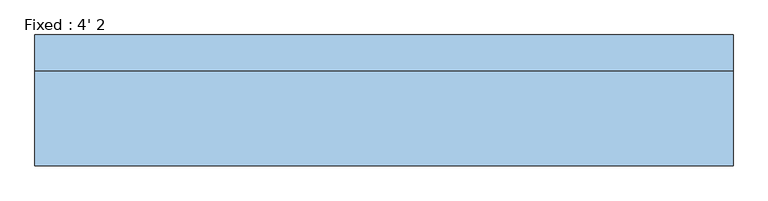
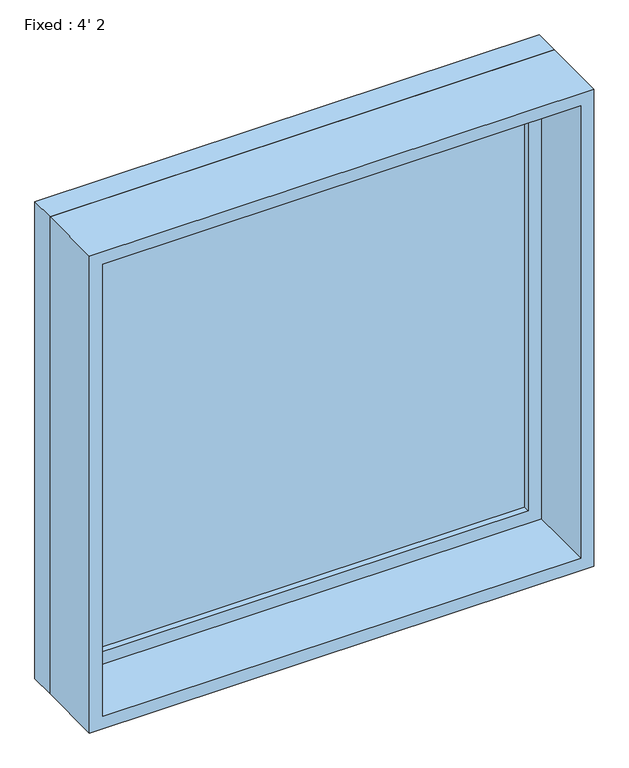
"""IFC4 building model written with IfcOpenShell, lengths in millimetres: window geometry, Fixed : 4' 2."""

from ifc_helpers import new_model, si_unit, frame, origin, place, context, project, spatial, polyline, outline, extrude, source, transform, mapped, element, save


def fixed_4_2_76f305d9(model_context):
    return source(origin(), model_context, "Body", "SweptSolid", [
        extrude(outline(polyline([(508.0, 66.675), (-584.2, 66.675), (-584.2, 79.375), (508.0, 79.375), (508.0, 66.675)])), frame((0.0, 0.0, 977.9), z_axis=(0.0, 0.0, 1.0), x_axis=(1.0, 0.0, 0.0)), (0.0, 0.0, 1.0), 1092.2),
        extrude(outline(polyline([(2114.55, -628.65), (933.45, -628.65), (933.45, 552.45), (2114.55, 552.45), (2114.55, -628.65)]), holes=[polyline([(2070.1, -584.2), (2070.1, 508.0), (977.9, 508.0), (977.9, -584.2), (2070.1, -584.2)])]), frame((0.0, 50.8, 0.0), z_axis=(0.0, 1.0, 0.0), x_axis=(0.0, 0.0, 1.0)), (0.0, 0.0, 1.0), 44.45),
        extrude(outline(polyline([(2133.6, -647.7), (914.4, -647.7), (914.4, 571.5), (2133.6, 571.5), (2133.6, -647.7)]), holes=[polyline([(2101.85, -615.95), (2101.85, 539.75), (946.15, 539.75), (946.15, -615.95), (2101.85, -615.95)])]), frame((0.0, -114.3, 0.0), z_axis=(0.0, 1.0, 0.0), x_axis=(0.0, 0.0, 1.0)), (0.0, 0.0, 1.0), 165.1),
        extrude(outline(polyline([(2133.6, 571.5), (2133.6, -647.7), (914.4, -647.7), (914.4, 571.5), (2133.6, 571.5)]), holes=[polyline([(2114.55, 552.45), (933.45, 552.45), (933.45, -628.65), (2114.55, -628.65), (2114.55, 552.45)])]), frame((0.0, 50.8, 0.0), z_axis=(0.0, 1.0, 0.0), x_axis=(0.0, 0.0, 1.0)), (0.0, 0.0, 1.0), 63.5),
    ])


if __name__ == "__main__":
    model = new_model("IFC4")
    model_context = context("Model", 3, world=origin())
    ifc_project = project(units=[si_unit("LENGTHUNIT", "METRE", prefix="MILLI")], contexts=[model_context])
    site = spatial("IfcSite", under=ifc_project)
    building = spatial("IfcBuilding", under=site)
    placement = place(None, origin())
    fixed_4_2_shape = fixed_4_2_76f305d9(model_context)
    element("IfcWindow", 1, ObjectType="Fixed : 4' 2", at=placement, inside=building, context=model_context, shape_type="MappedRepresentation", body=[
        mapped(fixed_4_2_shape, transform((0.0, 0.0, 0.0), x_axis=(1.0, 0.0, 0.0), y_axis=(0.0, 1.0, 0.0), z_axis=(0.0, 0.0, 1.0))),
    ])
    save(model, "model.ifc")

# Revit data of these elements
# Type "Fixed : 4' 2"
#   Type Mark = "20"
#   Construction Type Id = "GSP4R"
#   Assembly Code = "B2020100"
#   Analytic Construction = "1/8 in Pilkington single glazing"
#   Visual Light Transmittance = 0.9
#   Solar Heat Gain Coefficient = 0.78
#   Heat Transfer Coefficient (U) = 0.6496 BTU/(h·ft²·°F)
#   Height = 4' - 0"
#   Default Sill Height = 3' - 0"
#   Width = 4' - 0"
#   Window Inset = 0' - 0 3/4"
#   Define Thermal Properties by = 1
#   Glass Pane Material = Glass
#   Sash Material = Sash
#   Wall Closure = (empty or 0)
# Element 1 (IfcWindow, "Fixed : 4' 2")
#   Materials on its faces: "Sash", "Glass"
# Materials
#   "Glass": class "Glass", colour RGB 0 128 192, transparency 0.75, Description = "Soda Lime Glass", Cost = 0
#   "Sash": class "Wood", colour RGB 224 178 126, transparency 0, Cost = 0
